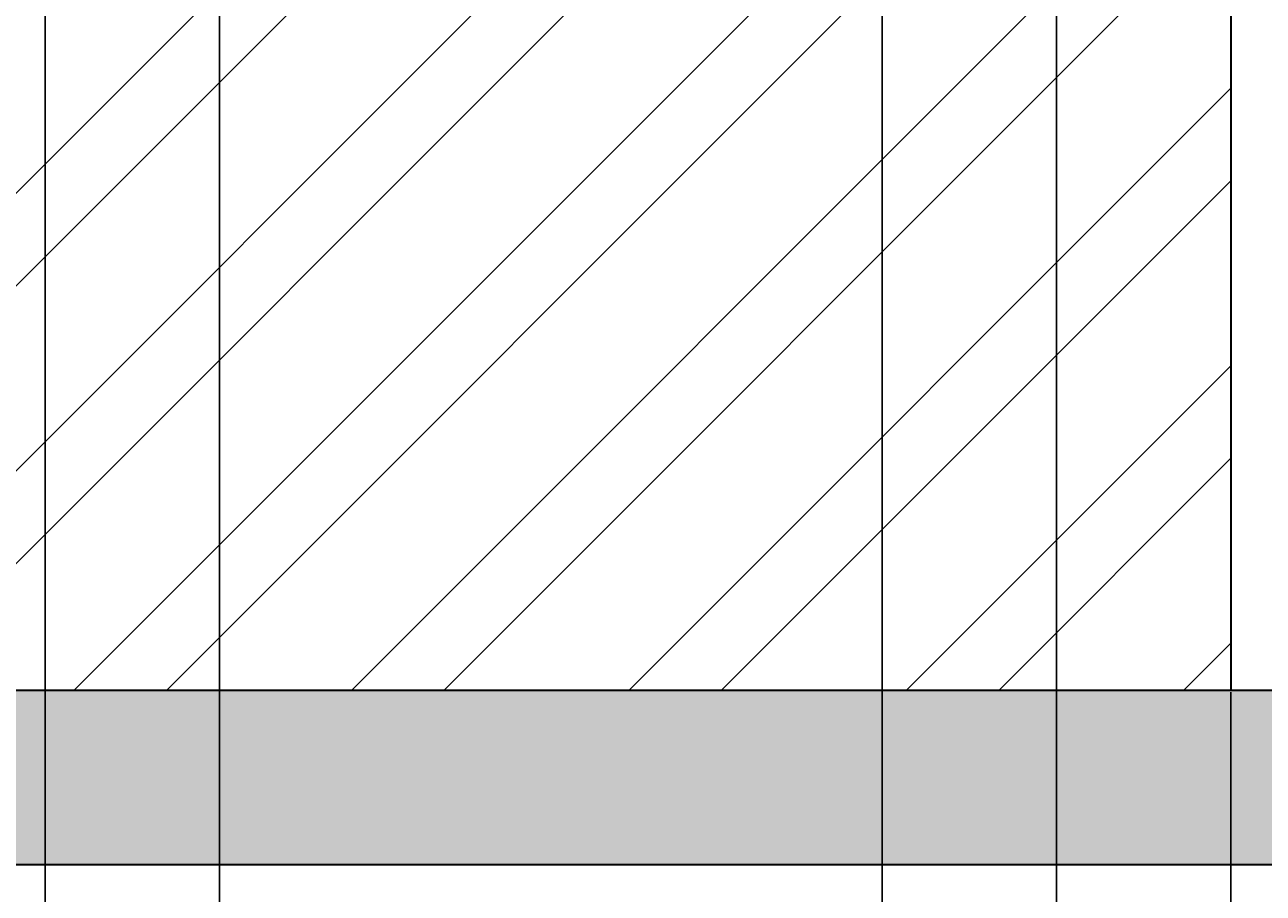
# Model space of a CAD drawing. Units: inches. Extents: x -301 to 715, y -607 to 364.
# Tile 30 of 141: x 124 to 159, y -541 to -516. Entities that reach past the tile are written whole.
import ezdxf

# ---------------------------------------------------------------- set-up
doc = ezdxf.new("R2010")
doc.units = ezdxf.units.IN
doc.header["$MEASUREMENT"] = 0
for name, color, linetype, lineweight in [('A-ANNO-DIMS', 2, 'Continuous', 18), ('A-SECT-PATT', 8, 'Continuous', 13), ('S-FNDN', 2, 'Continuous', 35)]:
    doc.layers.add(name, color=color, linetype=linetype, lineweight=lineweight)
doc.styles.get("Standard").update_dxf_attribs({"font": 'arial.ttf'})
doc.dimstyles.get("Standard").update_dxf_attribs({"dimtxt": 0.18, "dimasz": 0.18, "dimexe": 0.18, "dimexo": 0.0625, "dimgap": 0.09, "dimtad": 0, "dimtih": 1, "dimtoh": 1, "dimdec": 1, "dimzin": 0, "dimdsep": 46, "dimlunit": 4, "dimtxsty": 'Standard', "dimcen": 0.09, "dimclrd": 3, "dimclre": 4, "dimclrt": 6, "dimadec": 0, "dimazin": 0, "dimtfac": 1, "dimtdec": 1, "dimtofl": 0, "dimtmove": 0, "dimatfit": 3, "dimfxl": 1, "dimtfill": 2, "dimtfillclr": 51, "dimtolj": 1, "dimtzin": 0, "dimarcsym": 0})

# ---------------------------------------------------------------- blocks, each defined once
blk = doc.blocks.new('*D78')
at = {"layer": 'A-ANNO-DIMS', "color": 0, "lineweight": -2, "transparency": 16777216}
for p, q in [((158.318, -511.477), (177.276, -511.477)), ((177.096, -516.477), (177.096, -520.877)), ((177.096, -530.477), (177.096, -526.078)), ((158.318, -535.477), (177.276, -535.477))]:
    blk.add_line(p, q, dxfattribs=at)
at = {"layer": 'A-ANNO-DIMS', "color": 0, "transparency": 16777216}
for points in [[(176.262, -516.477), (177.929, -516.477), (177.096, -511.477)], [(176.262, -530.477), (177.929, -530.477), (177.096, -535.477)]]:
    blk.add_solid(points, dxfattribs=at)
at = {"layer": 'Defpoints', "color": 0, "transparency": 16777216}
for p in [(158.255, -511.477), (177.096, -511.477), (158.255, -535.477)]:
    blk.add_point(p, dxfattribs=at)
at = {"layer": 'A-ANNO-DIMS', "color": 0, "transparency": 16777216, "insert": (177.096, -523.477), "char_height": 5, "attachment_point": 5, "bg_fill": 1, "box_fill_scale": 1.25, "bg_fill_color": 51, "bg_fill_transparency": 0}
blk.add_mtext("\\A1;2'", dxfattribs=at)
blk = doc.blocks.new('*D176')
at = {"layer": 'A-ANNO-DIMS', "color": 4, "lineweight": -2, "transparency": 16777216}
for p, q in [((148.28, -324.477), (215.605, -324.477)), ((-15.22, -540.477), (215.605, -540.477))]:
    blk.add_line(p, q, dxfattribs=at)
at = {"layer": 'A-ANNO-DIMS', "color": 3, "lineweight": -2, "transparency": 16777216}
for p, q in [((215.425, -324.657), (215.425, -432.296)), ((215.425, -540.297), (215.425, -432.659))]:
    blk.add_line(p, q, dxfattribs=at)
at = {"layer": 'A-ANNO-DIMS', "color": 3, "transparency": 16777216}
for points in [[(215.395, -324.657), (215.455, -324.657), (215.425, -324.477)], [(215.395, -540.297), (215.455, -540.297), (215.425, -540.477)]]:
    blk.add_solid(points, dxfattribs=at)
at = {"layer": 'Defpoints', "color": 0, "transparency": 16777216}
for p in [(148.218, -324.477), (-15.282, -540.477), (215.425, -540.477)]:
    blk.add_point(p, dxfattribs=at)
at = {"layer": 'A-ANNO-DIMS', "color": 6, "transparency": 16777216, "insert": (215.425, -432.477), "char_height": 0.18, "attachment_point": 5, "bg_fill": 1, "box_fill_scale": 1.25, "bg_fill_color": 51, "bg_fill_transparency": 0}
blk.add_mtext('\\A1;18\'-0"', dxfattribs=at)
blk = doc.blocks.new('*D182')
at = {"layer": 'A-ANNO-DIMS', "color": 4, "lineweight": -2, "transparency": 16777216}
for p, q in [((114.255, -540.54), (114.255, -573.809)), ((163.255, -540.54), (163.255, -573.809))]:
    blk.add_line(p, q, dxfattribs=at)
at = {"layer": 'A-ANNO-DIMS', "color": 3, "lineweight": -2, "transparency": 16777216}
for p, q in [((114.435, -573.629), (138.422, -573.629)), ((163.075, -573.629), (139.088, -573.629))]:
    blk.add_line(p, q, dxfattribs=at)
at = {"layer": 'A-ANNO-DIMS', "color": 3, "transparency": 16777216}
for points in [[(114.435, -573.599), (114.435, -573.659), (114.255, -573.629)], [(163.075, -573.599), (163.075, -573.659), (163.255, -573.629)]]:
    blk.add_solid(points, dxfattribs=at)
at = {"layer": 'Defpoints', "color": 0, "transparency": 16777216}
for p in [(114.255, -540.477), (163.255, -540.477), (163.255, -573.629)]:
    blk.add_point(p, dxfattribs=at)
at = {"layer": 'A-ANNO-DIMS', "color": 6, "transparency": 16777216, "insert": (138.755, -573.629), "char_height": 0.18, "attachment_point": 5, "bg_fill": 1, "box_fill_scale": 1.25, "bg_fill_color": 51, "bg_fill_transparency": 0}
blk.add_mtext('\\A1;4\'-1"', dxfattribs=at)
blk = doc.blocks.new('*D183')
at = {"layer": 'A-ANNO-DIMS', "color": 4, "lineweight": -2, "transparency": 16777216}
for p, q in [((119.255, -535.54), (119.255, -573.809)), ((158.255, -535.54), (158.255, -573.809))]:
    blk.add_line(p, q, dxfattribs=at)
at = {"layer": 'A-ANNO-DIMS', "color": 3, "lineweight": -2, "transparency": 16777216}
for p, q in [((119.435, -573.629), (138.426, -573.629)), ((158.075, -573.629), (139.084, -573.629))]:
    blk.add_line(p, q, dxfattribs=at)
at = {"layer": 'A-ANNO-DIMS', "color": 3, "transparency": 16777216}
for points in [[(119.435, -573.599), (119.435, -573.659), (119.255, -573.629)], [(158.075, -573.599), (158.075, -573.659), (158.255, -573.629)]]:
    blk.add_solid(points, dxfattribs=at)
at = {"layer": 'Defpoints', "color": 0, "transparency": 16777216}
for p in [(119.255, -535.477), (158.255, -535.477), (158.255, -573.629)]:
    blk.add_point(p, dxfattribs=at)
at = {"layer": 'A-ANNO-DIMS', "color": 6, "transparency": 16777216, "insert": (138.755, -573.629), "char_height": 0.18, "attachment_point": 5, "bg_fill": 1, "box_fill_scale": 1.25, "bg_fill_color": 51, "bg_fill_transparency": 0}
blk.add_mtext('\\A1;3\'-3"', dxfattribs=at)
blk = doc.blocks.new('*D184')
at = {"layer": 'A-ANNO-DIMS', "color": 4, "lineweight": -2, "transparency": 16777216}
for p, q in [((124.255, -511.54), (124.255, -573.809)), ((153.255, -511.54), (153.255, -573.809))]:
    blk.add_line(p, q, dxfattribs=at)
at = {"layer": 'A-ANNO-DIMS', "color": 3, "lineweight": -2, "transparency": 16777216}
for p, q in [((124.435, -573.629), (138.424, -573.629)), ((153.075, -573.629), (139.086, -573.629))]:
    blk.add_line(p, q, dxfattribs=at)
at = {"layer": 'A-ANNO-DIMS', "color": 3, "transparency": 16777216}
for points in [[(124.435, -573.599), (124.435, -573.659), (124.255, -573.629)], [(153.075, -573.599), (153.075, -573.659), (153.255, -573.629)]]:
    blk.add_solid(points, dxfattribs=at)
at = {"layer": 'Defpoints', "color": 0, "transparency": 16777216}
for p in [(124.255, -511.477), (153.255, -511.477), (153.255, -573.629)]:
    blk.add_point(p, dxfattribs=at)
at = {"layer": 'A-ANNO-DIMS', "color": 6, "transparency": 16777216, "insert": (138.755, -573.629), "char_height": 0.18, "attachment_point": 5, "bg_fill": 1, "box_fill_scale": 1.25, "bg_fill_color": 51, "bg_fill_transparency": 0}
blk.add_mtext('\\A1;2\'-5"', dxfattribs=at)
blk = doc.blocks.new('*D185')
at = {"layer": 'A-ANNO-DIMS', "color": 4, "lineweight": -2, "transparency": 16777216}
for p, q in [((129.255, -493.54), (129.255, -573.809)), ((148.255, -493.54), (148.255, -573.809))]:
    blk.add_line(p, q, dxfattribs=at)
at = {"layer": 'A-ANNO-DIMS', "color": 3, "lineweight": -2, "transparency": 16777216}
for p, q in [((129.435, -573.629), (138.434, -573.629)), ((148.075, -573.629), (139.076, -573.629))]:
    blk.add_line(p, q, dxfattribs=at)
at = {"layer": 'A-ANNO-DIMS', "color": 3, "transparency": 16777216}
for points in [[(129.435, -573.599), (129.435, -573.659), (129.255, -573.629)], [(148.075, -573.599), (148.075, -573.659), (148.255, -573.629)]]:
    blk.add_solid(points, dxfattribs=at)
at = {"layer": 'Defpoints', "color": 0, "transparency": 16777216}
for p in [(129.255, -493.477), (148.255, -493.477), (148.255, -573.629)]:
    blk.add_point(p, dxfattribs=at)
at = {"layer": 'A-ANNO-DIMS', "color": 6, "transparency": 16777216, "insert": (138.755, -573.629), "char_height": 0.18, "attachment_point": 5, "bg_fill": 1, "box_fill_scale": 1.25, "bg_fill_color": 51, "bg_fill_transparency": 0}
blk.add_mtext('\\A1;1\'-7"', dxfattribs=at)
blk = doc.blocks.new('*D191')
at = {"layer": 'A-ANNO-DIMS', "color": 4, "lineweight": -2, "transparency": 16777216}
for p, q in [((129.193, -481.477), (-266.112, -481.477)), ((114.193, -540.477), (-266.112, -540.477))]:
    blk.add_line(p, q, dxfattribs=at)
at = {"layer": 'A-ANNO-DIMS', "color": 3, "lineweight": -2, "transparency": 16777216}
for p, q in [((-265.932, -481.657), (-265.932, -510.797)), ((-265.932, -540.297), (-265.932, -511.158))]:
    blk.add_line(p, q, dxfattribs=at)
at = {"layer": 'A-ANNO-DIMS', "color": 3, "transparency": 16777216}
for points in [[(-265.962, -481.657), (-265.902, -481.657), (-265.932, -481.477)], [(-265.962, -540.297), (-265.902, -540.297), (-265.932, -540.477)]]:
    blk.add_solid(points, dxfattribs=at)
at = {"layer": 'Defpoints', "color": 0, "transparency": 16777216}
for p in [(129.255, -481.477), (-265.932, -540.477), (114.255, -540.477)]:
    blk.add_point(p, dxfattribs=at)
at = {"layer": 'A-ANNO-DIMS', "color": 6, "transparency": 16777216, "insert": (-265.932, -510.977), "char_height": 0.18, "attachment_point": 5, "bg_fill": 1, "box_fill_scale": 1.25, "bg_fill_color": 51, "bg_fill_transparency": 0}
blk.add_mtext('\\A1;4\'-11"', dxfattribs=at)

msp = doc.modelspace()

# ---------------------------------------------------------------- hatches: boundary and pattern name
at = {"layer": 'A-SECT-PATT'}
h = msp.add_hatch(dxfattribs=at)
h.set_pattern_fill('ANSI32', color=256, scale=15)
h.set_pattern_definition([(45, (10.321, 33.8764), (-3.977476, 3.977476), []), (45, (12.973, 33.8764), (-3.977476, 3.977476), [])])
h.paths.add_polyline_path([(-185.282, -324.477), (-199.282, -324.477), (-199.282, -329.477), (-194.282, -329.477), (-194.282, -353.477), (-185.282, -353.477)])
h.paths.add_polyline_path([(-185.282, -361.477), (-193.904, -361.477), (-193.982, -377.537), (-185.282, -377.537)])
h.paths.add_polyline_path([(143.218, -329.477), (148.218, -329.477), (148.218, -324.477), (134.255, -324.477), (134.255, -353.477), (143.218, -353.477)])
h.paths.add_polyline_path([(143.218, -361.477), (134.255, -361.477), (134.255, -377.477), (143.218, -377.477)])
h.paths.add_polyline_path([(-185.282, -439.477), (-194.282, -439.477), (-194.282, -463.477), (-185.282, -463.477)])
h.paths.add_polyline_path([(-185.282, -471.477), (-194.282, -471.477), (-194.282, -481.477), (-185.282, -481.477)])
h.paths.add_polyline_path([(-185.282, -463.477), (-194.282, -463.477), (-194.282, -466.477), (-185.282, -466.477)])
h.paths.add_polyline_path([(-185.282, -466.477), (-194.282, -466.477), (-194.282, -471.477), (-185.282, -471.477)])
h.paths.add_polyline_path([(-180.282, -481.477), (-185.282, -481.477), (-194.282, -481.477), (-199.282, -481.477), (-199.282, -493.477), (-180.282, -493.477)])
h.paths.add_polyline_path([(-175.282, -493.477), (-180.282, -493.477), (-199.282, -493.477), (-204.282, -493.477), (-204.282, -511.477), (-175.282, -511.477)])
h.paths.add_polyline_path([(-170.282, -511.477), (-175.282, -511.477), (-204.282, -511.477), (-209.282, -511.477), (-209.282, -535.477), (-170.282, -535.477)])
h.paths.add_polyline_path([(-35.282, -463.477), (-41.282, -463.477), (-41.282, -466.477), (-35.282, -466.477)])
h.paths.add_polyline_path([(-35.282, -466.477), (-41.282, -466.477), (-41.282, -471.477), (-35.282, -471.477)])
h.paths.add_polyline_path([(-35.282, -471.477), (-41.282, -471.477), (-41.282, -481.477), (-35.282, -481.477)])
h.paths.add_polyline_path([(-30.282, -481.477), (-46.282, -481.477), (-46.282, -493.477), (-30.282, -493.477)])
h.paths.add_polyline_path([(-25.282, -493.477), (-30.282, -493.477), (-46.282, -493.477), (-51.282, -493.477), (-51.282, -511.477), (-25.282, -511.477)])
h.paths.add_polyline_path([(-20.282, -511.477), (-25.282, -511.477), (-51.282, -511.477), (-56.282, -511.477), (-56.282, -535.477), (-20.282, -535.477)])
h.paths.add_polyline_path([(143.218, -463.477), (134.255, -463.477), (134.255, -466.477), (143.218, -466.477)])
h.paths.add_polyline_path([(143.218, -466.477), (134.255, -466.477), (134.255, -471.477), (143.218, -471.477)])
h.paths.add_polyline_path([(143.218, -471.477), (134.255, -471.477), (134.255, -481.477), (143.218, -481.477)])
h.paths.add_polyline_path([(148.255, -481.477), (143.255, -481.477), (134.255, -481.477), (129.255, -481.477), (129.255, -493.477), (148.255, -493.477)])
h.paths.add_polyline_path([(153.255, -493.477), (148.255, -493.477), (129.255, -493.477), (124.255, -493.477), (124.255, -511.477), (153.255, -511.477)])
h.paths.add_polyline_path([(158.255, -511.477), (153.255, -511.477), (124.255, -511.477), (119.255, -511.477), (119.255, -535.477), (158.255, -535.477)])
h = msp.add_hatch(dxfattribs=at)
h.set_pattern_fill('AR-CONC', color=256, scale=0.5)
h.set_pattern_definition([(50, (10.3213, 33.8764), (3.586301, -0.31376), [0.375, -4.125]), (355, (10.3213, 33.8764), (-0.693757, 3.76096), [0.3, -3.3]), (100.45144, (10.62, 33.8502), (2.892544, 3.4472), [0.3187, -3.50571]), (46.1842, (10.3213, 34.8764), (5.336207, -0.827596), [0.5625, -6.1875]), (96.6356, (10.766, 34.8074), (4.67331, 4.870593), [0.47805, -5.25857]), (351.1842, (10.321, 34.8764), (4.67331, 4.870593), [0.45, -4.95]), (21, (10.8213, 34.6264), (2.984535, -2.013094), [0.375, -4.125]), (326, (10.8213, 34.6264), (1.216577, 3.62575), [0.3, -3.3]), (71.45144, (11.07, 34.4586), (4.201112, 1.612656), [0.3187, -3.50571]), (37.5, (10.3213, 33.8764), (0.0607993, 1.6644693), [0, -3.26, 0, -3.35, 0, -3.3125]), (7.5, (10.3213, 33.8764), (1.3153477, 1.9720586), [0, -1.91, 0, -3.185, 0, -1.2625]), (327.5, (9.2063, 33.8764), (2.6691122, -0.1127744), [0, -1.25, 0, -3.9, 0, -5.175]), (317.5, (8.7063, 33.8764), (2.915931, 0.500525), [0, -1.625, 0, -2.59, 0, -3.675])])
h.paths.add_polyline_path([(-56.282, -535.477), (-61.282, -535.477), (-61.282, -540.477), (-15.282, -540.477), (-15.282, -535.477), (-20.282, -535.477)])
h.paths.add_polyline_path([(119.255, -535.477), (114.255, -535.477), (114.255, -540.477), (163.255, -540.477), (163.255, -535.477), (158.255, -535.477)])
h.paths.add_polyline_path([(-206.282, -471.477), (-209.282, -471.477), (-209.282, -481.477), (-206.282, -481.477), (-194.282, -481.477), (-194.282, -471.477)])
h.paths.add_polyline_path([(-41.282, -481.477), (-41.282, -471.477), (-185.282, -471.477), (-185.282, -481.477), (-180.282, -481.477)])
h.paths.add_polyline_path([(134.255, -481.477), (134.255, -471.477), (-35.282, -471.477), (-35.282, -481.477), (-30.282, -481.477)])
h.paths.add_polyline_path([(155.218, -481.477), (158.218, -481.477), (158.218, -471.477), (153.218, -471.477), (143.218, -471.477), (143.218, -481.477), (148.255, -481.477)])
h.paths.add_polyline_path([(-193.88, -356.477), (-193.904, -361.477), (143.218, -361.477), (143.218, -356.477)])

# ---------------------------------------------------------------- linework, layer by layer
at = {"layer": 'S-FNDN'}
for p, q in [((158.255, -511.477), (158.255, -535.477)), ((119.255, -535.477), (158.255, -535.477)), ((158.255, -535.477), (163.255, -535.477)), ((114.255, -540.477), (163.255, -540.477))]:
    msp.add_line(p, q, dxfattribs=at)

# ---------------------------------------------------------------- dimensions: what is measured, and where the dimension line sits
at = {"layer": 'A-ANNO-DIMS'}
for base, p1, p2, override, picture, middle in [((215.425, -540.477), (148.218, -324.477), (-15.282, -540.477), {"dimdec": 1, "dimlfac": 1, "dimrnd": 0, "dimzin": 1, "dimdsep": 46, "dimlunit": 4, "dimfrac": 2}, '*D176', (215.425, -432.477)), ((-265.932, -540.477), (129.255, -481.477), (114.255, -540.477), {"dimdec": 1, "dimlfac": 1, "dimrnd": 0, "dimzin": 1, "dimdsep": 46, "dimlunit": 4, "dimfrac": 2}, '*D191', (-265.932, -510.977)), ((177.096, -511.477), (158.255, -535.477), (158.255, -511.477), {"dimtxt": 5, "dimasz": 5, "dimclrd": 0, "dimclre": 0, "dimclrt": 0}, '*D78', (177.096, -523.477))]:
    dim = msp.add_linear_dim(base=base, p1=p1, p2=p2, angle=90, dimstyle='Standard', override=override, dxfattribs=at)
    dim.commit()
    dim.dimension.update_dxf_attribs({"geometry": picture, "text_midpoint": middle})
for base, p1, p2, picture in [((148.255, -573.629), (129.255, -493.477), (148.255, -493.477), '*D185'), ((153.255, -573.629), (124.255, -511.477), (153.255, -511.477), '*D184'), ((158.255, -573.629), (119.255, -535.477), (158.255, -535.477), '*D183'), ((163.255, -573.629), (114.255, -540.477), (163.255, -540.477), '*D182')]:
    dim = msp.add_linear_dim(base=base, p1=p1, p2=p2, dimstyle='Standard', override={"dimdec": 1, "dimlfac": 1, "dimrnd": 0, "dimzin": 1, "dimdsep": 46, "dimlunit": 4, "dimfrac": 2}, dxfattribs=at)
    dim.commit()
    dim.dimension.update_dxf_attribs({"geometry": picture, "text_midpoint": (138.755, -573.629)})

doc.saveas('drawing.dxf')
